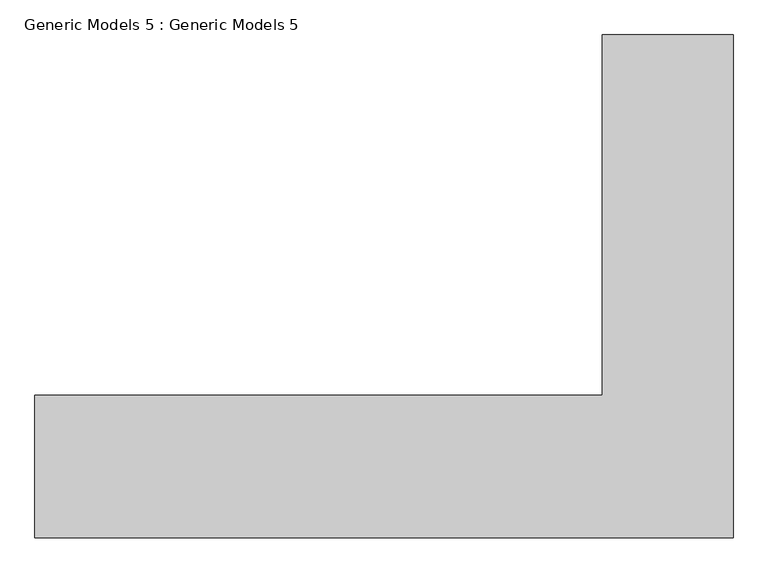
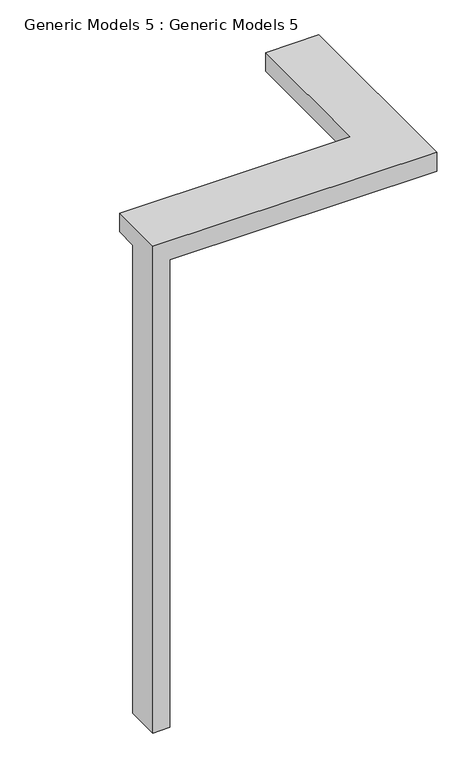
"""IFC4 building model written with IfcOpenShell, lengths in millimetres: proxy geometry, Generic Models 5 : Generic Models 5."""

from ifc_helpers import new_model, si_unit, origin, place, context, project, spatial, faceted_brep, source, transform, mapped, element, save


def generic_models_5_generic_models_5_9540ccd6(model_context):
    return source(origin(), model_context, "Body", "Brep", [
        faceted_brep([(-9743.0321088, -5738.2962979, 11420.6045332), (-10894.660896, -5738.2962979, 11420.6045332), (-10894.660896, -8905.1468404, 11420.6045332), (-15877.1321088, -8905.1468404, 11420.6045332), (-15877.1321088, -10154.3940225, 11420.6045332), (-9743.0321088, -10154.3940225, 11420.6045332), (-9743.0321088, -10154.3940225, 10988.8045332), (-15512.0003513, -10154.3940225, 10988.8045332), (-15512.0003513, -9400.4468404, 10988.8045332), (-15877.1321088, -9400.4468404, 10988.8045332), (-15877.1321088, -8905.1468404, 10988.8045332), (-10894.660896, -8905.1468404, 10988.8045332), (-10894.660896, -5738.2962979, 10988.8045332), (-9743.0321088, -5738.2962979, 10988.8045332), (-15877.1321088, -9400.4468404, 304.8), (-15877.1321088, -10154.3940225, 304.8), (-15512.0003513, -10154.3940225, 304.8), (-15512.0003513, -9400.4468404, 304.8)], [[[0, 1, 2, 3, 4, 5]], [[6, 7, 8, 9, 10, 11, 12, 13]], [[0, 5, 6, 13]], [[10, 3, 2, 11]], [[4, 3, 10, 9, 14, 15]], [[5, 4, 15, 16, 7, 6]], [[14, 9, 8, 17]], [[16, 15, 14, 17]], [[7, 16, 17, 8]], [[1, 0, 13, 12]], [[2, 1, 12, 11]]]),
    ])


if __name__ == "__main__":
    model = new_model("IFC4")
    model_context = context("Model", 3, world=origin())
    ifc_project = project(units=[si_unit("LENGTHUNIT", "METRE", prefix="MILLI")], contexts=[model_context])
    site = spatial("IfcSite", under=ifc_project)
    building = spatial("IfcBuilding", under=site)
    placement = place(None, origin())
    generic_models_5_generic_models_5_shape = generic_models_5_generic_models_5_9540ccd6(model_context)
    element("IfcBuildingElementProxy", 1, Name="Generic Models 5 : Generic Models 5", ObjectType="Generic Models 5 : Generic Models 5", at=placement, inside=building, context=model_context, shape_type="MappedRepresentation", body=[
        mapped(generic_models_5_generic_models_5_shape, transform((0.0, 0.0, 0.0), x_axis=(1.0, 0.0, 0.0), y_axis=(0.0, 1.0, 0.0), z_axis=(0.0, 0.0, 1.0))),
    ])
    save(model, "model.ifc")
